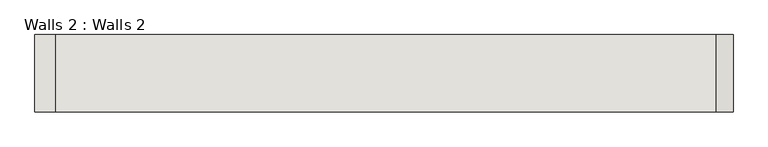
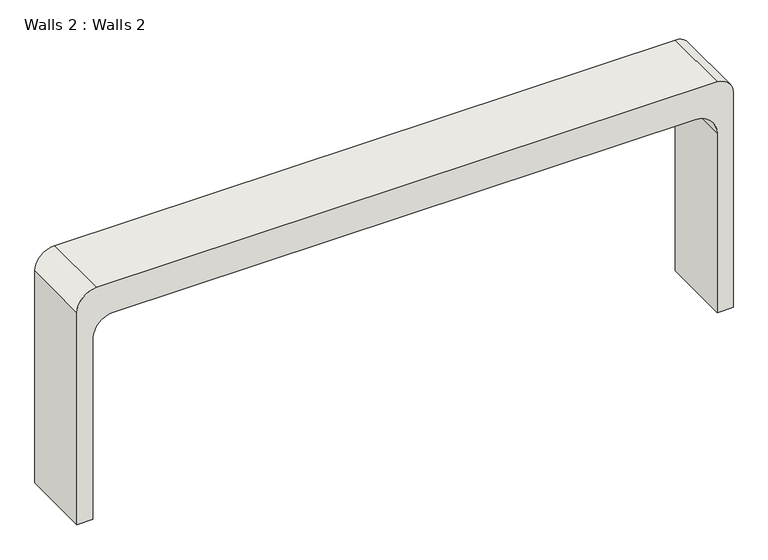
"""IFC4 building model written with IfcOpenShell, lengths in millimetres: wall geometry, Walls 2 : Walls 2."""

from ifc_helpers import new_model, si_unit, point, frame, frame_2d, origin, place, context, project, spatial, polyline, circle_curve, trimmed, segment, composite_curve, outline, extrude, source, transform, mapped, element, save


def walls_2_walls_2_336146d7(model_context):
    return source(origin(), model_context, "Body", "SweptSolid", [
        extrude(outline(composite_curve([segment(polyline([(8896.4, 3660.4261575), (6096.0, 3660.4261575), (6096.0, 3860.4261575), (8490.0, 3860.4261575)]), True, "CONTINUOUS"), segment(trimmed(circle_curve(frame_2d((8490.0, 4114.4261575)), 254.0), [point((8490.0, 3860.4261575))], [point((8744.0, 4114.4261575))], True, "CARTESIAN"), True, "CONTINUOUS"), segment(polyline([(8744.0, 4114.4261575), (8744.0, 11382.3023789)]), True, "CONTINUOUS"), segment(trimmed(circle_curve(frame_2d((8464.6, 11382.3023789)), 279.4), [point((8744.0, 11382.3023789))], [point((8464.6, 11661.7023789))], True, "CARTESIAN"), True, "CONTINUOUS"), segment(polyline([(8464.6, 11661.7023789), (6096.0, 11661.7023789), (6096.0, 11861.7023789), (8944.0, 11861.7023789)]), True, "CONTINUOUS"), segment(trimmed(circle_curve(frame_2d((8944.0, 11661.7023789)), 200.0), [point((8944.0, 11861.7023789))], [point((9144.0, 11661.7023789))], False, "CARTESIAN"), True, "CONTINUOUS"), segment(polyline([(9144.0, 11661.7023789), (9144.0, 3908.0261575)]), True, "CONTINUOUS"), segment(trimmed(circle_curve(frame_2d((8896.4, 3908.0261575)), 247.6), [point((9144.0, 3908.0261575))], [point((8896.4, 3660.4261575))], False, "CARTESIAN"), True, "CONTINUOUS")], self_intersect=False)), frame((0.0, -4049.3114058, 0.0), z_axis=(0.0, 1.0, 0.0), x_axis=(0.0, 0.0, 1.0)), (0.0, 0.0, 1.0), 910.5603133),
    ])


if __name__ == "__main__":
    model = new_model("IFC4")
    model_context = context("Model", 3, world=origin())
    ifc_project = project(units=[si_unit("LENGTHUNIT", "METRE", prefix="MILLI")], contexts=[model_context])
    site = spatial("IfcSite", under=ifc_project)
    building = spatial("IfcBuilding", under=site)
    placement = place(None, origin())
    walls_2_walls_2_shape = walls_2_walls_2_336146d7(model_context)
    element("IfcWall", 1, ObjectType="Walls 2 : Walls 2", at=placement, inside=building, context=model_context, shape_type="MappedRepresentation", body=[
        mapped(walls_2_walls_2_shape, transform((0.0, 0.0, 0.0), x_axis=(1.0, 0.0, 0.0), y_axis=(0.0, 1.0, 0.0), z_axis=(0.0, 0.0, 1.0))),
    ])
    save(model, "model.ifc")

# Revit data of these elements
# Element 1 (IfcWall, "Walls 2 : Walls 2")
#   Materials on its faces: "Default Wall"
# Materials
#   "Default Wall": colour RGB 80 80 80, transparency 0
